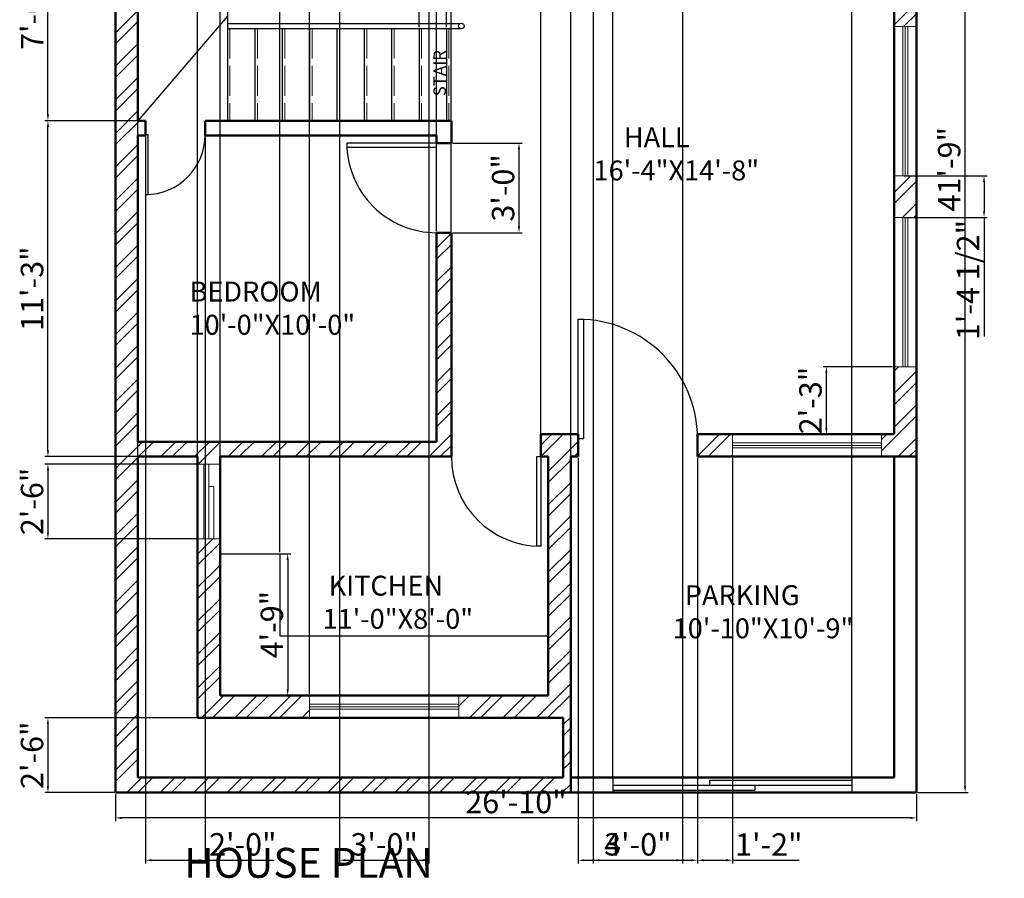
# Model space of a CAD drawing. Units: inches. Extents: x 234 to 630, y 1038 to 1631.
# Tile 1 of 2: x 234 to 630, y 1038 to 1383. Entities that reach past the tile are written whole.
import ezdxf

# ---------------------------------------------------------------- set-up
doc = ezdxf.new("R2010")
doc.units = ezdxf.units.IN
doc.linetypes.add('ACAD_ISO02W100', pattern=[15, 12, -3])
for name, color, linetype, lineweight in [('A-ANNO-DIMS', 2, 'Continuous', 18), ('A-ANNO-TEXT', 7, 'Continuous', 35), ('A-AREA-IDEN', 7, 'Continuous', 25), ('A-DOOR', 4, 'Continuous', 25), ('A-FLOR-FIXT', 8, 'Continuous', 25), ('A-FLOR-STRS', 7, 'Continuous', 25), ('A-FLOR-STRS-HIDN', 8, 'ACAD_ISO02W100', 13), ('A-GLAZ', 244, 'Continuous', 18), ('A-WALL', 7, 'Continuous', 50), ('A-WALL-PATT', 252, 'Continuous', 13)]:
    doc.layers.add(name, color=color, linetype=linetype, lineweight=lineweight)
doc.styles.get("Standard").update_dxf_attribs({"font": 'arial.ttf'})
doc.dimstyles.new('ISO-25', dxfattribs={"dimtxt": 9, "dimasz": 2.5, "dimexe": 1.25, "dimexo": 0.625, "dimtad": 1, "dimlunit": 3, "dimtxsty": 'Standard', "dimcen": 2.5, "dimadec": 0, "dimazin": 0, "dimtfac": 1, "dimtmove": 0, "dimatfit": 3, "dimfxl": 1, "dimarcsym": 0})

# ---------------------------------------------------------------- blocks, each defined once
blk = doc.blocks.new('*U2')
for p, q in [((0, 0), (0, -6)), ((40, 0), (40, -6))]:
    blk.add_line(p, q)
blk.add_lwpolyline([(0, 0), (0, 40), (1.75, 40), (1.75, 0)], close=True)
blk.add_arc((0, 0), 40, 0, 90)
blk = doc.blocks.new('*U3')
for p, q in [((0, 0), (0, 6)), ((40, 0), (40, 6))]:
    blk.add_line(p, q)
blk.add_lwpolyline([(0, 0), (0, -40), (1.75, -40), (1.75, 0)], close=True)
blk.add_arc((0, 0), 40, 270, 0)
blk = doc.blocks.new('*U6')
for p, q in [((-40, 0), (-40, 6)), ((0, 0), (0, 6))]:
    blk.add_line(p, q)
blk.add_lwpolyline([(0, 0), (0, -40), (-1.75, -40), (-1.75, 0)], close=True)
blk.add_arc((0, 0), 40, 180, 270)
blk = doc.blocks.new('*U7')
for p, q in [((0, 0), (0, 6)), ((40, 0), (40, 6))]:
    blk.add_line(p, q)
blk.add_lwpolyline([(0, 0), (0, -40), (1.75, -40), (1.75, 0)], close=True)
blk.add_arc((0, 0), 40, 270, 0)
blk = doc.blocks.new('*D8')
at = {"layer": 'A-ANNO-DIMS', "color": 0, "lineweight": -2, "transparency": 16777216}
for p, q in [((272.93, 1071.55), (272.93, 1060.74)), ((594.93, 1071.55), (594.93, 1060.74)), ((592.43, 1061.99), (275.43, 1061.99))]:
    blk.add_line(p, q, dxfattribs=at)
at = {"layer": 'A-ANNO-DIMS', "color": 0, "transparency": 16777216}
for points in [[(275.43, 1062.41), (275.43, 1061.58), (272.93, 1061.99)], [(592.43, 1062.41), (592.43, 1061.58), (594.93, 1061.99)]]:
    blk.add_solid(points, dxfattribs=at)
at = {"layer": 'Defpoints', "color": 0, "transparency": 16777216}
for p in [(272.93, 1072.18), (594.93, 1072.18), (272.93, 1061.99)]:
    blk.add_point(p, dxfattribs=at)
at = {"layer": 'A-ANNO-DIMS', "color": 0, "transparency": 16777216, "insert": (433.93, 1067.21), "char_height": 9, "attachment_point": 5}
blk.add_mtext('26\'-10"', dxfattribs=at)
blk = doc.blocks.new('*D9')
at = {"layer": 'A-ANNO-DIMS', "color": 0, "lineweight": -2, "transparency": 16777216}
for p, q in [((595.56, 1573.18), (615.76, 1573.18)), ((614.51, 1074.68), (614.51, 1570.68)), ((595.56, 1072.18), (615.76, 1072.18))]:
    blk.add_line(p, q, dxfattribs=at)
at = {"layer": 'A-ANNO-DIMS', "color": 0, "transparency": 16777216}
for points in [[(614.09, 1570.68), (614.92, 1570.68), (614.51, 1573.18)], [(614.09, 1074.68), (614.92, 1074.68), (614.51, 1072.18)]]:
    blk.add_solid(points, dxfattribs=at)
at = {"layer": 'Defpoints', "color": 0, "transparency": 16777216}
for p in [(594.93, 1573.18), (614.51, 1573.18), (594.93, 1072.18)]:
    blk.add_point(p, dxfattribs=at)
at = {"layer": 'A-ANNO-DIMS', "color": 0, "transparency": 16777216, "insert": (609.29, 1322.68), "char_height": 9, "attachment_point": 5, "rotation": 90}
blk.add_mtext('41\'-9"', dxfattribs=at)
blk = doc.blocks.new('WIN-GLAZING-60IN')
for p, q in [((0, 2), (60, 2)), ((0, 1), (60, 1)), ((0, 0), (60, 0))]:
    blk.add_line(p, q)
blk = doc.blocks.new('*D16')
at = {"layer": 'A-ANNO-DIMS', "color": 0, "lineweight": -2, "transparency": 16777216}
for p, q in [((281.31, 1426.18), (244.48, 1426.18)), ((245.73, 1344.68), (245.73, 1423.68)), ((281.31, 1342.18), (244.48, 1342.18))]:
    blk.add_line(p, q, dxfattribs=at)
at = {"layer": 'A-ANNO-DIMS', "color": 0, "transparency": 16777216}
for points in [[(245.31, 1423.68), (246.15, 1423.68), (245.73, 1426.18)], [(245.31, 1344.68), (246.15, 1344.68), (245.73, 1342.18)]]:
    blk.add_solid(points, dxfattribs=at)
at = {"layer": 'Defpoints', "color": 0, "transparency": 16777216}
for p in [(245.73, 1426.18), (281.93, 1426.18), (281.93, 1342.18)]:
    blk.add_point(p, dxfattribs=at)
at = {"layer": 'A-ANNO-DIMS', "color": 0, "transparency": 16777216, "insert": (240.51, 1384.18), "char_height": 9, "attachment_point": 5, "rotation": 90}
blk.add_mtext('7\'-0"', dxfattribs=at)
blk = doc.blocks.new('*D17')
at = {"layer": 'A-ANNO-DIMS', "color": 0, "lineweight": -2, "transparency": 16777216}
for p, q in [((281.31, 1342.18), (244.48, 1342.18)), ((245.73, 1209.68), (245.73, 1339.68)), ((281.31, 1207.18), (244.48, 1207.18))]:
    blk.add_line(p, q, dxfattribs=at)
at = {"layer": 'A-ANNO-DIMS', "color": 0, "transparency": 16777216}
for points in [[(245.31, 1339.68), (246.15, 1339.68), (245.73, 1342.18)], [(245.31, 1209.68), (246.15, 1209.68), (245.73, 1207.18)]]:
    blk.add_solid(points, dxfattribs=at)
at = {"layer": 'Defpoints', "color": 0, "transparency": 16777216}
for p in [(245.73, 1342.18), (281.93, 1342.18), (281.93, 1207.18)]:
    blk.add_point(p, dxfattribs=at)
at = {"layer": 'A-ANNO-DIMS', "color": 0, "transparency": 16777216, "insert": (240.51, 1274.68), "char_height": 9, "attachment_point": 5, "rotation": 90}
blk.add_mtext('11\'-3"', dxfattribs=at)
blk = doc.blocks.new('*D20')
at = {"layer": 'A-ANNO-DIMS', "color": 0, "lineweight": -2, "transparency": 16777216}
for p, q in [((585.31, 1243.3), (557.48, 1243.3)), ((558.73, 1218.68), (558.73, 1240.8)), ((585.31, 1216.18), (557.48, 1216.18))]:
    blk.add_line(p, q, dxfattribs=at)
at = {"layer": 'A-ANNO-DIMS', "color": 0, "transparency": 16777216}
for points in [[(558.31, 1240.8), (559.15, 1240.8), (558.73, 1243.3)], [(558.31, 1218.68), (559.15, 1218.68), (558.73, 1216.18)]]:
    blk.add_solid(points, dxfattribs=at)
at = {"layer": 'Defpoints', "color": 0, "transparency": 16777216}
for p in [(558.73, 1243.3), (585.93, 1243.3), (585.93, 1216.18)]:
    blk.add_point(p, dxfattribs=at)
at = {"layer": 'A-ANNO-DIMS', "color": 0, "transparency": 16777216, "insert": (553.51, 1229.74), "char_height": 9, "attachment_point": 5, "rotation": 90}
blk.add_mtext('2\'-3"', dxfattribs=at)
blk = doc.blocks.new('*D21')
at = {"layer": 'A-ANNO-DIMS', "color": 0, "lineweight": -2, "transparency": 16777216}
for p, q in [((590.06, 1320.04), (623.38, 1320.04)), ((622.13, 1317.54), (622.13, 1305.8)), ((590.06, 1303.3), (623.38, 1303.3)), ((622.13, 1303.3), (622.13, 1255.5))]:
    blk.add_line(p, q, dxfattribs=at)
at = {"layer": 'A-ANNO-DIMS', "color": 0, "transparency": 16777216}
for points in [[(621.71, 1317.54), (622.55, 1317.54), (622.13, 1320.04)], [(621.71, 1305.8), (622.55, 1305.8), (622.13, 1303.3)]]:
    blk.add_solid(points, dxfattribs=at)
at = {"layer": 'Defpoints', "color": 0, "transparency": 16777216}
for p in [(589.43, 1320.04), (589.43, 1303.3), (622.13, 1303.3)]:
    blk.add_point(p, dxfattribs=at)
at = {"layer": 'A-ANNO-DIMS', "color": 0, "transparency": 16777216, "insert": (616.85, 1278.15), "char_height": 9, "attachment_point": 5, "rotation": 90}
blk.add_mtext('1\'-4 1/2"', dxfattribs=at)
blk = doc.blocks.new('*D22')
at = {"layer": 'A-ANNO-DIMS', "color": 0, "lineweight": -2, "transparency": 16777216}
for p, q in [((281.93, 1078.8), (281.93, 1601.63)), ((284.43, 1600.38), (303.43, 1600.38)), ((305.93, 1102.8), (305.93, 1601.63)), ((305.93, 1600.38), (333.76, 1600.38))]:
    blk.add_line(p, q, dxfattribs=at)
at = {"layer": 'A-ANNO-DIMS', "color": 0, "transparency": 16777216}
for points in [[(284.43, 1600.8), (284.43, 1599.96), (281.93, 1600.38)], [(303.43, 1600.8), (303.43, 1599.96), (305.93, 1600.38)]]:
    blk.add_solid(points, dxfattribs=at)
at = {"layer": 'Defpoints', "color": 0, "transparency": 16777216}
for p in [(305.93, 1600.38), (305.93, 1102.18), (281.93, 1078.18)]:
    blk.add_point(p, dxfattribs=at)
at = {"layer": 'A-ANNO-DIMS', "color": 0, "transparency": 16777216, "insert": (321.09, 1605.6), "char_height": 9, "attachment_point": 5}
blk.add_mtext('2\'-0"', dxfattribs=at)
blk = doc.blocks.new('*D23')
at = {"layer": 'A-ANNO-DIMS', "color": 0, "lineweight": -2, "transparency": 16777216}
for p, q in [((305.31, 1102.18), (244.48, 1102.18)), ((245.73, 1099.68), (245.73, 1074.68)), ((272.31, 1072.18), (244.48, 1072.18))]:
    blk.add_line(p, q, dxfattribs=at)
at = {"layer": 'A-ANNO-DIMS', "color": 0, "transparency": 16777216}
for points in [[(245.31, 1099.68), (246.15, 1099.68), (245.73, 1102.18)], [(245.31, 1074.68), (246.15, 1074.68), (245.73, 1072.18)]]:
    blk.add_solid(points, dxfattribs=at)
at = {"layer": 'Defpoints', "color": 0, "transparency": 16777216}
for p in [(305.93, 1102.18), (245.73, 1072.18), (272.93, 1072.18)]:
    blk.add_point(p, dxfattribs=at)
at = {"layer": 'A-ANNO-DIMS', "color": 0, "transparency": 16777216, "insert": (240.51, 1087.18), "char_height": 9, "attachment_point": 5, "rotation": 90}
blk.add_mtext('2\'-6"', dxfattribs=at)
blk = doc.blocks.new('*D24')
at = {"layer": 'A-ANNO-DIMS', "color": 0, "lineweight": -2, "transparency": 16777216}
for p, q in [((472.93, 1078.8), (472.93, 1601.63)), ((475.43, 1600.38), (566.43, 1600.38)), ((568.93, 1078.8), (568.93, 1601.63))]:
    blk.add_line(p, q, dxfattribs=at)
at = {"layer": 'A-ANNO-DIMS', "color": 0, "transparency": 16777216}
for points in [[(475.43, 1600.8), (475.43, 1599.96), (472.93, 1600.38)], [(566.43, 1600.8), (566.43, 1599.96), (568.93, 1600.38)]]:
    blk.add_solid(points, dxfattribs=at)
at = {"layer": 'Defpoints', "color": 0, "transparency": 16777216}
for p in [(568.93, 1600.38), (472.93, 1078.18), (568.93, 1078.18)]:
    blk.add_point(p, dxfattribs=at)
at = {"layer": 'A-ANNO-DIMS', "color": 0, "transparency": 16777216, "insert": (520.93, 1605.6), "char_height": 9, "attachment_point": 5}
blk.add_mtext('8\'-0"', dxfattribs=at)
blk = doc.blocks.new('*D25')
at = {"layer": 'A-ANNO-DIMS', "color": 0, "lineweight": -2, "transparency": 16777216}
for p, q in [((455.93, 1078.8), (455.93, 1601.63)), ((458.43, 1600.38), (470.43, 1600.38)), ((472.93, 1078.8), (472.93, 1601.63)), ((472.93, 1600.38), (499.76, 1600.38))]:
    blk.add_line(p, q, dxfattribs=at)
at = {"layer": 'A-ANNO-DIMS', "color": 0, "transparency": 16777216}
for points in [[(458.43, 1600.8), (458.43, 1599.96), (455.93, 1600.38)], [(470.43, 1600.8), (470.43, 1599.96), (472.93, 1600.38)]]:
    blk.add_solid(points, dxfattribs=at)
at = {"layer": 'Defpoints', "color": 0, "transparency": 16777216}
for p in [(472.93, 1600.38), (455.93, 1078.18), (472.93, 1078.18)]:
    blk.add_point(p, dxfattribs=at)
at = {"layer": 'A-ANNO-DIMS', "color": 0, "transparency": 16777216, "insert": (487.59, 1605.6), "char_height": 9, "attachment_point": 5}
blk.add_mtext('1\'-5"', dxfattribs=at)
blk = doc.blocks.new('*D26')
at = {"layer": 'A-ANNO-DIMS', "color": 0, "lineweight": -2, "transparency": 16777216}
for p, q in [((458.93, 1206.55), (458.93, 1043.73)), ((506.93, 1206.55), (506.93, 1043.73)), ((461.43, 1044.98), (504.43, 1044.98))]:
    blk.add_line(p, q, dxfattribs=at)
at = {"layer": 'A-ANNO-DIMS', "color": 0, "transparency": 16777216}
for points in [[(461.43, 1045.4), (461.43, 1044.56), (458.93, 1044.98)], [(504.43, 1045.4), (504.43, 1044.56), (506.93, 1044.98)]]:
    blk.add_solid(points, dxfattribs=at)
at = {"layer": 'Defpoints', "color": 0, "transparency": 16777216}
for p in [(458.93, 1207.18), (506.93, 1207.18), (506.93, 1044.98)]:
    blk.add_point(p, dxfattribs=at)
at = {"layer": 'A-ANNO-DIMS', "color": 0, "transparency": 16777216, "insert": (482.93, 1050.2), "char_height": 9, "attachment_point": 5}
blk.add_mtext('4\'-0"', dxfattribs=at)
blk = doc.blocks.new('*D27')
at = {"layer": 'A-ANNO-DIMS', "color": 0, "lineweight": -2, "transparency": 16777216}
for p, q in [((506.93, 1206.55), (506.93, 1043.73)), ((520.93, 1206.55), (520.93, 1043.73)), ((509.43, 1044.98), (518.43, 1044.98)), ((520.93, 1044.98), (547.76, 1044.98))]:
    blk.add_line(p, q, dxfattribs=at)
at = {"layer": 'A-ANNO-DIMS', "color": 0, "transparency": 16777216}
for points in [[(509.43, 1045.4), (509.43, 1044.56), (506.93, 1044.98)], [(518.43, 1045.4), (518.43, 1044.56), (520.93, 1044.98)]]:
    blk.add_solid(points, dxfattribs=at)
at = {"layer": 'Defpoints', "color": 0, "transparency": 16777216}
for p in [(506.93, 1207.18), (520.93, 1207.18), (520.93, 1044.98)]:
    blk.add_point(p, dxfattribs=at)
at = {"layer": 'A-ANNO-DIMS', "color": 0, "transparency": 16777216, "insert": (535.59, 1050.12), "char_height": 9, "attachment_point": 5}
blk.add_mtext('1\'-2"', dxfattribs=at)
blk = doc.blocks.new('*D28')
at = {"layer": 'A-ANNO-DIMS', "color": 0, "lineweight": -2, "transparency": 16777216}
for p, q in [((407.93, 1207.8), (407.93, 1601.63)), ((410.43, 1600.38), (441.43, 1600.38)), ((443.93, 1207.8), (443.93, 1601.63))]:
    blk.add_line(p, q, dxfattribs=at)
at = {"layer": 'A-ANNO-DIMS', "color": 0, "transparency": 16777216}
for points in [[(410.43, 1600.8), (410.43, 1599.96), (407.93, 1600.38)], [(441.43, 1600.8), (441.43, 1599.96), (443.93, 1600.38)]]:
    blk.add_solid(points, dxfattribs=at)
at = {"layer": 'Defpoints', "color": 0, "transparency": 16777216}
for p in [(443.93, 1600.38), (407.93, 1207.18), (443.93, 1207.18)]:
    blk.add_point(p, dxfattribs=at)
at = {"layer": 'A-ANNO-DIMS', "color": 0, "transparency": 16777216, "insert": (425.93, 1605.6), "char_height": 9, "attachment_point": 5}
blk.add_mtext('3\'-0"', dxfattribs=at)
blk = doc.blocks.new('*D29')
at = {"layer": 'A-ANNO-DIMS', "color": 0, "lineweight": -2, "transparency": 16777216}
for p, q in [((314.93, 1111.8), (314.93, 1601.63)), ((317.43, 1600.38), (348.43, 1600.38)), ((350.93, 1111.8), (350.93, 1601.63))]:
    blk.add_line(p, q, dxfattribs=at)
at = {"layer": 'A-ANNO-DIMS', "color": 0, "transparency": 16777216}
for points in [[(317.43, 1600.8), (317.43, 1599.96), (314.93, 1600.38)], [(348.43, 1600.8), (348.43, 1599.96), (350.93, 1600.38)]]:
    blk.add_solid(points, dxfattribs=at)
at = {"layer": 'Defpoints', "color": 0, "transparency": 16777216}
for p in [(350.93, 1600.38), (314.93, 1111.18), (350.93, 1111.18)]:
    blk.add_point(p, dxfattribs=at)
at = {"layer": 'A-ANNO-DIMS', "color": 0, "transparency": 16777216, "insert": (332.93, 1605.6), "char_height": 9, "attachment_point": 5}
blk.add_mtext('3\'-0"', dxfattribs=at)
blk = doc.blocks.new('*D30')
at = {"layer": 'A-ANNO-DIMS', "color": 0, "lineweight": -2, "transparency": 16777216}
for p, q in [((314.93, 1168.81), (314.93, 1601.63)), ((317.43, 1600.38), (336.43, 1600.38)), ((338.93, 1168.81), (338.93, 1601.63)), ((338.93, 1600.38), (366.76, 1600.38))]:
    blk.add_line(p, q, dxfattribs=at)
at = {"layer": 'A-ANNO-DIMS', "color": 0, "transparency": 16777216}
for points in [[(317.43, 1600.8), (317.43, 1599.96), (314.93, 1600.38)], [(336.43, 1600.8), (336.43, 1599.96), (338.93, 1600.38)]]:
    blk.add_solid(points, dxfattribs=at)
at = {"layer": 'Defpoints', "color": 0, "transparency": 16777216}
for p in [(338.93, 1600.38), (314.93, 1168.18), (338.93, 1168.18)]:
    blk.add_point(p, dxfattribs=at)
at = {"layer": 'A-ANNO-DIMS', "color": 0, "transparency": 16777216, "insert": (354.09, 1605.6), "char_height": 9, "attachment_point": 5}
blk.add_mtext('2\'-0"', dxfattribs=at)
blk = doc.blocks.new('*D31')
at = {"layer": 'A-ANNO-DIMS', "color": 0, "lineweight": -2, "transparency": 16777216}
for p, q in [((305.31, 1204.18), (244.48, 1204.18)), ((245.73, 1201.68), (245.73, 1176.68)), ((305.31, 1174.18), (244.48, 1174.18))]:
    blk.add_line(p, q, dxfattribs=at)
at = {"layer": 'A-ANNO-DIMS', "color": 0, "transparency": 16777216}
for points in [[(245.31, 1201.68), (246.15, 1201.68), (245.73, 1204.18)], [(245.31, 1176.68), (246.15, 1176.68), (245.73, 1174.18)]]:
    blk.add_solid(points, dxfattribs=at)
at = {"layer": 'Defpoints', "color": 0, "transparency": 16777216}
for p in [(305.93, 1204.18), (245.73, 1174.18), (305.93, 1174.18)]:
    blk.add_point(p, dxfattribs=at)
at = {"layer": 'A-ANNO-DIMS', "color": 0, "transparency": 16777216, "insert": (240.51, 1189.18), "char_height": 9, "attachment_point": 5, "rotation": 90}
blk.add_mtext('2\'-6"', dxfattribs=at)
blk = doc.blocks.new('*D32')
at = {"layer": 'A-ANNO-DIMS', "color": 0, "lineweight": -2, "transparency": 16777216}
for p, q in [((399.43, 1600.38), (396.93, 1600.38)), ((401.93, 1297.8), (401.93, 1601.63)), ((401.93, 1600.38), (407.93, 1600.38)), ((407.93, 1297.8), (407.93, 1601.63)), ((410.43, 1600.38), (438.1, 1600.38))]:
    blk.add_line(p, q, dxfattribs=at)
at = {"layer": 'A-ANNO-DIMS', "color": 0, "transparency": 16777216}
for points in [[(399.43, 1600.8), (399.43, 1599.96), (401.93, 1600.38)], [(410.43, 1600.8), (410.43, 1599.96), (407.93, 1600.38)]]:
    blk.add_solid(points, dxfattribs=at)
at = {"layer": 'Defpoints', "color": 0, "transparency": 16777216}
for p in [(407.93, 1600.38), (401.93, 1297.18), (407.93, 1297.18)]:
    blk.add_point(p, dxfattribs=at)
at = {"layer": 'A-ANNO-DIMS', "color": 0, "transparency": 16777216, "insert": (425.52, 1605.6), "char_height": 9, "attachment_point": 5}
blk.add_mtext('0\'-6"', dxfattribs=at)
blk = doc.blocks.new('*D34')
at = {"layer": 'A-ANNO-DIMS', "color": 0, "lineweight": -2, "transparency": 16777216}
for p, q in [((362.93, 1425.55), (362.93, 1043.73)), ((398.93, 1425.55), (398.93, 1043.73)), ((365.43, 1044.98), (396.43, 1044.98))]:
    blk.add_line(p, q, dxfattribs=at)
at = {"layer": 'A-ANNO-DIMS', "color": 0, "transparency": 16777216}
for points in [[(365.43, 1045.4), (365.43, 1044.56), (362.93, 1044.98)], [(396.43, 1045.4), (396.43, 1044.56), (398.93, 1044.98)]]:
    blk.add_solid(points, dxfattribs=at)
at = {"layer": 'Defpoints', "color": 0, "transparency": 16777216}
for p in [(362.93, 1426.18), (398.93, 1426.18), (398.93, 1044.98)]:
    blk.add_point(p, dxfattribs=at)
at = {"layer": 'A-ANNO-DIMS', "color": 0, "transparency": 16777216, "insert": (380.93, 1050.2), "char_height": 9, "attachment_point": 5}
blk.add_mtext('3\'-0"', dxfattribs=at)
blk = doc.blocks.new('*D35')
at = {"layer": 'A-ANNO-DIMS', "color": 0, "lineweight": -2, "transparency": 16777216}
for p, q in [((464.93, 1425.55), (464.93, 1043.73)), ((500.93, 1425.55), (500.93, 1043.73)), ((467.43, 1044.98), (498.43, 1044.98))]:
    blk.add_line(p, q, dxfattribs=at)
at = {"layer": 'A-ANNO-DIMS', "color": 0, "transparency": 16777216}
for points in [[(467.43, 1045.4), (467.43, 1044.56), (464.93, 1044.98)], [(498.43, 1045.4), (498.43, 1044.56), (500.93, 1044.98)]]:
    blk.add_solid(points, dxfattribs=at)
at = {"layer": 'Defpoints', "color": 0, "transparency": 16777216}
for p in [(464.93, 1426.18), (500.93, 1426.18), (500.93, 1044.98)]:
    blk.add_point(p, dxfattribs=at)
at = {"layer": 'A-ANNO-DIMS', "color": 0, "transparency": 16777216, "insert": (482.93, 1050.2), "char_height": 9, "attachment_point": 5}
blk.add_mtext('3\'-0"', dxfattribs=at)
blk = doc.blocks.new('*D38')
at = {"layer": 'A-ANNO-DIMS', "color": 0, "lineweight": -2, "transparency": 16777216}
for p, q in [((284.93, 1335.55), (284.93, 1043.73)), ((308.93, 1335.55), (308.93, 1043.73)), ((287.43, 1044.98), (306.43, 1044.98)), ((308.93, 1044.98), (336.76, 1044.98))]:
    blk.add_line(p, q, dxfattribs=at)
at = {"layer": 'A-ANNO-DIMS', "color": 0, "transparency": 16777216}
for points in [[(287.43, 1045.4), (287.43, 1044.56), (284.93, 1044.98)], [(306.43, 1045.4), (306.43, 1044.56), (308.93, 1044.98)]]:
    blk.add_solid(points, dxfattribs=at)
at = {"layer": 'Defpoints', "color": 0, "transparency": 16777216}
for p in [(284.93, 1336.18), (308.93, 1336.18), (308.93, 1044.98)]:
    blk.add_point(p, dxfattribs=at)
at = {"layer": 'A-ANNO-DIMS', "color": 0, "transparency": 16777216, "insert": (324.09, 1050.2), "char_height": 9, "attachment_point": 5}
blk.add_mtext('2\'-0"', dxfattribs=at)
blk = doc.blocks.new('*D39')
at = {"layer": 'A-ANNO-DIMS', "color": 0, "lineweight": -2, "transparency": 16777216}
for p, q in [((408.56, 1333.18), (436.38, 1333.18)), ((435.13, 1330.68), (435.13, 1299.68)), ((408.56, 1297.18), (436.38, 1297.18))]:
    blk.add_line(p, q, dxfattribs=at)
at = {"layer": 'A-ANNO-DIMS', "color": 0, "transparency": 16777216}
for points in [[(434.71, 1330.68), (435.55, 1330.68), (435.13, 1333.18)], [(434.71, 1299.68), (435.55, 1299.68), (435.13, 1297.18)]]:
    blk.add_solid(points, dxfattribs=at)
at = {"layer": 'Defpoints', "color": 0, "transparency": 16777216}
for p in [(407.93, 1333.18), (407.93, 1297.18), (435.13, 1297.18)]:
    blk.add_point(p, dxfattribs=at)
at = {"layer": 'A-ANNO-DIMS', "color": 0, "transparency": 16777216, "insert": (429.91, 1315.18), "char_height": 9, "attachment_point": 5, "rotation": 90}
blk.add_mtext('3\'-0"', dxfattribs=at)
blk = doc.blocks.new('*D40')
at = {"layer": 'A-ANNO-DIMS', "color": 0, "lineweight": -2, "transparency": 16777216}
for p, q in [((394.93, 1379.8), (394.93, 1407.63)), ((397.43, 1406.38), (403.43, 1406.38)), ((405.93, 1379.8), (405.93, 1407.63)), ((405.93, 1406.38), (440.6, 1406.38))]:
    blk.add_line(p, q, dxfattribs=at)
at = {"layer": 'A-ANNO-DIMS', "color": 0, "transparency": 16777216}
for points in [[(397.43, 1406.8), (397.43, 1405.96), (394.93, 1406.38)], [(403.43, 1406.8), (403.43, 1405.96), (405.93, 1406.38)]]:
    blk.add_solid(points, dxfattribs=at)
at = {"layer": 'Defpoints', "color": 0, "transparency": 16777216}
for p in [(405.93, 1406.38), (394.93, 1379.18), (405.93, 1379.18)]:
    blk.add_point(p, dxfattribs=at)
at = {"layer": 'A-ANNO-DIMS', "color": 0, "transparency": 16777216, "insert": (424.51, 1411.6), "char_height": 9, "attachment_point": 5}
blk.add_mtext('0\'-11"', dxfattribs=at)
blk = doc.blocks.new('*D42')
at = {"layer": 'A-ANNO-DIMS', "color": 0, "lineweight": -2, "transparency": 16777216}
for p, q in [((315.56, 1168.18), (343.38, 1168.18)), ((342.13, 1165.68), (342.13, 1113.68)), ((315.56, 1111.18), (343.38, 1111.18))]:
    blk.add_line(p, q, dxfattribs=at)
at = {"layer": 'A-ANNO-DIMS', "color": 0, "transparency": 16777216}
for points in [[(341.71, 1165.68), (342.55, 1165.68), (342.13, 1168.18)], [(341.71, 1113.68), (342.55, 1113.68), (342.13, 1111.18)]]:
    blk.add_solid(points, dxfattribs=at)
at = {"layer": 'Defpoints', "color": 0, "transparency": 16777216}
for p in [(314.93, 1168.18), (314.93, 1111.18), (342.13, 1111.18)]:
    blk.add_point(p, dxfattribs=at)
at = {"layer": 'A-ANNO-DIMS', "color": 0, "transparency": 16777216, "insert": (336.91, 1139.68), "char_height": 9, "attachment_point": 5, "rotation": 90}
blk.add_mtext('4\'-9"', dxfattribs=at)

msp = doc.modelspace()

# ---------------------------------------------------------------- hatches: boundary and pattern name
at = {"layer": 'A-WALL-PATT'}
h = msp.add_hatch(dxfattribs=at)
h.set_pattern_fill('ANSI32', color=256)
h.paths.add_polyline_path([(407.931, 1216.178), (407.931, 1297.178), (401.931, 1297.178), (401.931, 1213.178), (281.931, 1213.178), (281.931, 1336.178), (284.931, 1336.178), (284.931, 1342.178), (281.931, 1342.178), (281.931, 1426.178), (362.931, 1426.178), (362.931, 1432.178), (281.931, 1432.178), (281.931, 1564.178), (311.931, 1564.178), (311.931, 1573.178), (272.931, 1573.178), (272.931, 1072.178), (455.931, 1072.178), (455.931, 1102.178), (455.931, 1207.178), (458.931, 1207.178), (458.931, 1216.178), (443.931, 1216.178), (443.931, 1207.178), (446.931, 1207.178), (446.931, 1111.178), (410.931, 1111.178), (410.931, 1102.178), (452.931, 1102.178), (452.931, 1078.178), (281.931, 1078.178), (281.931, 1207.178), (305.931, 1207.178), (305.931, 1204.178), (314.931, 1204.178), (314.931, 1207.178), (407.931, 1207.178)])
h.paths.add_polyline_path([(314.931, 1174.178), (305.931, 1174.178), (305.931, 1102.178), (350.931, 1102.178), (350.931, 1111.178), (314.931, 1111.178)], flags=17)
h.paths.add_polyline_path([(493.931, 1573.178), (371.931, 1573.178), (371.931, 1564.178), (401.931, 1564.178), (401.931, 1492.178), (407.931, 1492.178), (407.931, 1495.178), (455.931, 1495.178), (455.931, 1432.178), (407.931, 1432.178), (407.931, 1462.178), (401.931, 1462.178), (401.931, 1432.178), (398.931, 1432.178), (398.931, 1426.178), (464.931, 1426.178), (464.931, 1432.178), (461.931, 1432.178), (461.931, 1504.178), (455.931, 1504.178), (455.931, 1501.178), (407.931, 1501.178), (407.931, 1564.178), (455.931, 1564.178), (455.931, 1534.178), (461.931, 1534.178), (461.931, 1564.178), (493.931, 1564.178)])
h.paths.add_polyline_path([(594.931, 1573.178), (553.931, 1573.178), (553.931, 1564.178), (585.931, 1564.178), (585.931, 1432.178), (500.931, 1432.178), (500.931, 1426.178), (585.931, 1426.178), (585.931, 1423.178), (594.931, 1423.178)])
h.paths.add_polyline_path([(594.931, 1320.043), (585.931, 1320.043), (585.931, 1303.302), (594.931, 1303.302)])
h.paths.add_polyline_path([(594.931, 1387.178), (585.931, 1387.178), (585.931, 1380.043), (594.931, 1380.043)])
h.paths.add_polyline_path([(594.931, 1243.302), (585.931, 1243.302), (585.931, 1216.178), (580.931, 1216.178), (580.931, 1207.178), (594.931, 1207.178)])
h.paths.add_polyline_path([(520.931, 1216.178), (506.931, 1216.178), (506.931, 1207.178), (520.931, 1207.178)])

# ---------------------------------------------------------------- linework, layer by layer
at = {"layer": 'A-DOOR'}
for p, q in [((472.931, 1078.178), (472.931, 1072.178)), ((511.931, 1077.178), (568.931, 1077.178)), ((511.931, 1075.178), (511.931, 1077.178)), ((568.931, 1078.178), (568.931, 1072.178)), ((472.931, 1075.178), (568.931, 1075.178)), ((472.931, 1073.178), (529.931, 1073.178)), ((529.931, 1075.178), (529.931, 1073.178))]:
    msp.add_line(p, q, dxfattribs=at)
at = {"layer": 'A-FLOR-FIXT'}
for p, q in [((314.931, 1168.185), (338.931, 1168.185)), ((338.931, 1168.185), (338.931, 1135.178)), ((338.931, 1135.178), (446.931, 1135.178))]:
    msp.add_line(p, q, dxfattribs=at)
at = {"layer": 'A-FLOR-STRS'}
for p, q in [((317.931, 1426.178), (317.931, 1342.178)), ((317.931, 1384.178), (281.931, 1342.178)), ((317.931, 1381.178), (411.353, 1381.178)), ((317.931, 1379.178), (411.55, 1379.178)), ((328.931, 1379.178), (328.931, 1342.178)), ((339.931, 1379.178), (339.931, 1342.178)), ((350.931, 1379.178), (350.931, 1342.178)), ((361.931, 1379.178), (361.931, 1342.178)), ((372.931, 1379.178), (372.931, 1342.178)), ((383.931, 1379.178), (383.931, 1342.178)), ((394.931, 1379.178), (394.931, 1342.178)), ((405.931, 1379.178), (405.931, 1342.178))]:
    msp.add_line(p, q, dxfattribs=at)
msp.add_circle((411.974, 1380.23), 1.134, dxfattribs=at)
at = {"layer": 'A-FLOR-STRS-HIDN'}
for p, q in [((318.931, 1379.178), (318.931, 1342.178)), ((329.931, 1379.178), (329.931, 1342.178)), ((340.931, 1379.178), (340.931, 1342.178)), ((351.931, 1379.178), (351.931, 1342.178)), ((362.931, 1379.178), (362.931, 1342.178)), ((373.931, 1379.178), (373.931, 1342.178)), ((384.931, 1379.178), (384.931, 1342.178)), ((395.931, 1379.178), (395.931, 1342.178)), ((406.931, 1379.178), (406.931, 1342.178))]:
    msp.add_line(p, q, dxfattribs=at)
at = {"layer": 'A-GLAZ'}
for p, q in [((314.931, 1204.178), (305.931, 1204.178)), ((308.431, 1204.178), (308.431, 1174.178)), ((310.431, 1204.178), (310.431, 1174.178)), ((310.431, 1195.178), (312.431, 1195.178)), ((312.431, 1195.178), (312.431, 1174.178)), ((314.931, 1174.178), (305.931, 1174.178))]:
    msp.add_line(p, q, dxfattribs=at)
for points in [[(594.931, 1380.043), (594.931, 1320.043), (585.931, 1320.043), (585.931, 1380.043)], [(594.931, 1303.302), (594.931, 1243.302), (585.931, 1243.302), (585.931, 1303.302)], [(520.931, 1216.178), (580.931, 1216.178), (580.931, 1207.178), (520.931, 1207.178)], [(350.931, 1111.178), (410.931, 1111.178), (410.931, 1102.178), (350.931, 1102.178)]]:
    msp.add_lwpolyline(points, close=True, dxfattribs=at)
at = {"layer": 'A-WALL'}
for p, q in [((272.931, 1573.178), (272.931, 1072.178)), ((281.931, 1426.178), (281.931, 1342.178)), ((585.931, 1387.178), (585.931, 1216.178)), ((594.931, 1387.178), (594.931, 1072.178)), ((281.931, 1342.178), (284.931, 1342.178)), ((284.931, 1336.178), (284.931, 1342.178)), ((308.931, 1336.178), (308.931, 1342.178)), ((308.931, 1342.178), (407.931, 1342.178)), ((407.931, 1342.178), (407.931, 1333.178)), ((281.931, 1336.178), (284.931, 1336.178)), ((281.931, 1336.178), (281.931, 1213.178)), ((308.931, 1336.178), (401.931, 1336.178)), ((401.931, 1336.178), (401.931, 1333.178)), ((401.931, 1333.178), (407.931, 1333.178)), ((401.931, 1297.178), (407.931, 1297.178)), ((401.931, 1297.178), (401.931, 1213.178)), ((407.931, 1297.178), (407.931, 1216.178)), ((407.931, 1207.178), (407.931, 1216.178)), ((443.931, 1216.178), (458.931, 1216.178)), ((443.931, 1207.178), (443.931, 1216.178)), ((458.931, 1207.178), (458.931, 1216.178)), ((506.931, 1207.178), (506.931, 1216.178)), ((506.931, 1216.178), (585.931, 1216.178)), ((281.931, 1213.178), (401.931, 1213.178)), ((281.931, 1207.178), (281.931, 1078.178)), ((281.931, 1207.178), (305.931, 1207.178)), ((305.931, 1207.178), (305.931, 1102.178)), ((314.931, 1207.178), (314.931, 1111.178)), ((314.931, 1207.178), (407.931, 1207.178)), ((443.931, 1207.178), (446.931, 1207.178)), ((446.931, 1207.178), (446.931, 1111.178)), ((455.931, 1207.178), (455.931, 1102.178)), ((455.931, 1207.178), (458.931, 1207.178)), ((506.931, 1207.178), (594.931, 1207.178)), ((585.931, 1207.178), (585.931, 1078.178)), ((314.931, 1111.178), (446.931, 1111.178)), ((305.931, 1102.178), (452.931, 1102.178)), ((452.931, 1102.178), (452.931, 1078.178)), ((455.931, 1102.178), (455.931, 1072.178)), ((281.931, 1078.178), (452.931, 1078.178)), ((455.931, 1078.178), (585.931, 1078.178)), ((272.931, 1072.178), (594.931, 1072.178))]:
    msp.add_line(p, q, dxfattribs=at)

# ---------------------------------------------------------------- block references
at = {"layer": 'A-DOOR'}
for name, p, xscale, yscale, zscale in [('*U7', (284.931, 1336.478), 0.5999999999999999, 0.5999999999999999, 0.5999999999999999), ('*U2', (458.931, 1214.378), 1.199999999999999, 1.199999999999999, 1.199999999999999), ('*U6', (443.931, 1207.178), 0.9, 0.9, 0.9)]:
    msp.add_blockref(name, p, dxfattribs=dict(at, xscale=xscale, yscale=yscale, zscale=zscale))
at = {"layer": 'A-DOOR', "xscale": 0.9, "yscale": 0.9, "zscale": 0.9, "rotation": 270}
msp.add_blockref('*U3', (401.931, 1333.178), dxfattribs=at)
at = {"layer": 'A-GLAZ', "rotation": 269.9999999999998}
for p in [(589.431, 1380.043), (589.431, 1303.302)]:
    msp.add_blockref('WIN-GLAZING-60IN', p, dxfattribs=at)
at = {"layer": 'A-GLAZ'}
for p in [(520.931, 1210.678), (350.931, 1105.678)]:
    msp.add_blockref('WIN-GLAZING-60IN', p, dxfattribs=at)

# ---------------------------------------------------------------- texts
at = {"layer": 'A-ANNO-TEXT', "insert": (300.494, 1049.938), "char_height": 12, "attachment_point": 1}
msp.add_mtext_dynamic_manual_height_columns('HOUSE PLAN', width=113.55139, gutter_width=12.5, heights=[0], dxfattribs=at)
at = {"layer": 'A-AREA-IDEN', "insert": (400.76, 1351.967), "char_height": 5, "attachment_point": 1, "rotation": 90}
msp.add_mtext_dynamic_manual_height_columns('STAIR', width=21.37669, gutter_width=12.5, heights=[2.72], dxfattribs=at)
at = {"layer": 'A-AREA-IDEN', "char_height": 8, "attachment_point": 1}
for s, width, insert in [('     HALL\\P16\'-4"X14\'-8"', 65.23778, (465.092, 1339.529)), ('BEDROOM\\P10\'-0"X10\'-0"', 65.23778, (302.68, 1277.515)), (' KITCHEN\\P11\'-0"X8\'-0"', 57.28847, (356.155, 1159.326)), ('  PARKING\\P10\'-10"X10\'-9"', 65.23778, (496.929, 1155.511))]:
    msp.add_mtext_dynamic_manual_height_columns(s, width=width, gutter_width=12.5, heights=[0], dxfattribs=dict(at, insert=insert))

# ---------------------------------------------------------------- dimensions: what is measured, and where the dimension line sits
at = {"layer": 'A-ANNO-DIMS'}
for base, p1, p2, override, picture, middle in [((305.931, 1600.378), (281.931, 1078.178), (305.931, 1102.178), {"dimdec": 1, "dimlfac": 1, "dimrnd": 0, "dimzin": 1, "dimdsep": 46, "dimlunit": 4, "dimfrac": 2}, '*D22', (321.094, 1605.599)), ((350.931, 1600.378), (314.931, 1111.178), (350.931, 1111.178), {"dimdec": 1, "dimlfac": 1, "dimrnd": 0, "dimzin": 1, "dimdsep": 46, "dimlunit": 4, "dimfrac": 2}, '*D29', (332.931, 1605.602)), ((338.931, 1600.378), (314.931, 1168.185), (338.931, 1168.185), {"dimdec": 1, "dimlfac": 1, "dimrnd": 0, "dimzin": 1, "dimdsep": 46, "dimlunit": 4, "dimfrac": 2}, '*D30', (354.094, 1605.599)), ((407.931, 1600.378), (401.931, 1297.178), (407.931, 1297.178), {"dimdec": 1, "dimlfac": 1, "dimrnd": 0, "dimzin": 1, "dimdsep": 46, "dimlunit": 4, "dimfrac": 2}, '*D32', (425.518, 1605.599)), ((443.931, 1600.378), (407.931, 1207.178), (443.931, 1207.178), {"dimdec": 1, "dimlfac": 1, "dimrnd": 0, "dimzin": 1, "dimdsep": 46, "dimlunit": 4, "dimfrac": 2}, '*D28', (425.931, 1605.602)), ((472.931, 1600.378), (455.931, 1078.178), (472.931, 1078.178), {"dimdec": 1, "dimlfac": 1, "dimrnd": 0, "dimzin": 1, "dimdsep": 46, "dimlunit": 4, "dimfrac": 2}, '*D25', (487.594, 1605.599)), ((568.931, 1600.378), (472.931, 1078.178), (568.931, 1078.178), {"dimdec": 1, "dimlfac": 1, "dimrnd": 0, "dimzin": 1, "dimdsep": 46, "dimlunit": 4, "dimfrac": 2}, '*D24', (520.931, 1605.599)), ((398.931, 1044.978), (362.931, 1426.178), (398.931, 1426.178), {"dimdec": 1, "dimlfac": 1, "dimrnd": 0, "dimzin": 1, "dimdsep": 46, "dimlunit": 4, "dimfrac": 2}, '*D34', (380.931, 1050.202)), ((500.931, 1044.978), (464.931, 1426.178), (500.931, 1426.178), {"dimdec": 1, "dimlfac": 1, "dimrnd": 0, "dimzin": 1, "dimdsep": 46, "dimlunit": 4, "dimfrac": 2}, '*D35', (482.931, 1050.202)), ((405.931, 1406.378), (394.931, 1379.178), (405.931, 1379.178), {"dimdec": 1, "dimlfac": 1, "dimrnd": 0, "dimzin": 1, "dimdsep": 46, "dimlunit": 4, "dimfrac": 2}, '*D40', (424.514, 1411.599)), ((308.931, 1044.978), (284.931, 1336.178), (308.931, 1336.178), {"dimdec": 1, "dimlfac": 1, "dimrnd": 0, "dimzin": 1, "dimdsep": 46, "dimlunit": 4, "dimfrac": 2}, '*D38', (324.094, 1050.199)), ((506.931, 1044.978), (458.931, 1207.178), (506.931, 1207.178), {"dimdec": 1, "dimlfac": 1, "dimrnd": 0, "dimzin": 1, "dimdsep": 46, "dimlunit": 4, "dimfrac": 2}, '*D26', (482.931, 1050.199)), ((520.931, 1044.978), (506.931, 1207.178), (520.931, 1207.178), {"dimdec": 1, "dimlfac": 1, "dimrnd": 0, "dimzin": 1, "dimdsep": 46, "dimlunit": 4, "dimfrac": 2}, '*D27', (535.594, 1050.122)), ((272.931, 1061.992), (594.931, 1072.178), (272.931, 1072.178), {"dimclrd": 0, "dimclre": 0, "dimclrt": 0}, '*D8', (433.931, 1067.212))]:
    dim = msp.add_linear_dim(base=base, p1=p1, p2=p2, dimstyle='ISO-25', override=override, dxfattribs=at)
    dim.commit()
    dim.dimension.update_dxf_attribs({"geometry": picture, "text_midpoint": middle})
for base, p1, p2, angle, override, picture, middle in [((614.506, 1573.178), (594.931, 1072.178), (594.931, 1573.178), 90, {"dimclrd": 0, "dimclre": 0, "dimclrt": 0}, '*D9', (609.286, 1322.678)), ((245.731, 1426.178), (281.931, 1342.178), (281.931, 1426.178), 90, {"dimdec": 1, "dimlfac": 1, "dimrnd": 0, "dimzin": 1, "dimdsep": 46, "dimlunit": 4, "dimfrac": 2}, '*D16', (240.51, 1384.178)), ((245.731, 1342.178), (281.931, 1207.178), (281.931, 1342.178), 90, {"dimdec": 1, "dimlfac": 1, "dimrnd": 0, "dimzin": 1, "dimdsep": 46, "dimlunit": 4, "dimfrac": 2}, '*D17', (240.507, 1274.678)), ((435.131, 1297.178), (407.931, 1333.178), (407.931, 1297.178), 270, {"dimdec": 1, "dimlfac": 1, "dimrnd": 0, "dimzin": 1, "dimdsep": 46, "dimlunit": 4, "dimfrac": 2}, '*D39', (429.907, 1315.178)), ((622.131, 1303.302), (589.431, 1320.043), (589.431, 1303.302), 90, {"dimdec": 1, "dimlfac": 1, "dimrnd": 0, "dimzin": 1, "dimdsep": 46, "dimlunit": 4, "dimfrac": 2}, '*D21', (616.852, 1278.152)), ((558.731, 1243.302), (585.931, 1216.178), (585.931, 1243.302), 90, {"dimdec": 1, "dimlfac": 1, "dimrnd": 0, "dimzin": 1, "dimdsep": 46, "dimlunit": 4, "dimfrac": 2}, '*D20', (553.507, 1229.74)), ((245.731, 1174.178), (305.931, 1204.178), (305.931, 1174.178), 90, {"dimdec": 1, "dimlfac": 1, "dimrnd": 0, "dimzin": 1, "dimdsep": 46, "dimlunit": 4, "dimfrac": 2}, '*D31', (240.51, 1189.178)), ((342.131, 1111.178), (314.931, 1168.185), (314.931, 1111.178), 270, {"dimdec": 1, "dimlfac": 1, "dimrnd": 0, "dimzin": 1, "dimdsep": 46, "dimlunit": 4, "dimfrac": 2}, '*D42', (336.91, 1139.682)), ((245.731, 1072.178), (305.931, 1102.178), (272.931, 1072.178), 90, {"dimdec": 1, "dimlfac": 1, "dimrnd": 0, "dimzin": 1, "dimdsep": 46, "dimlunit": 4, "dimfrac": 2}, '*D23', (240.51, 1087.178))]:
    dim = msp.add_linear_dim(base=base, p1=p1, p2=p2, angle=angle, dimstyle='ISO-25', override=override, dxfattribs=at)
    dim.commit()
    dim.dimension.update_dxf_attribs({"geometry": picture, "text_midpoint": middle})

doc.saveas('drawing.dxf')
